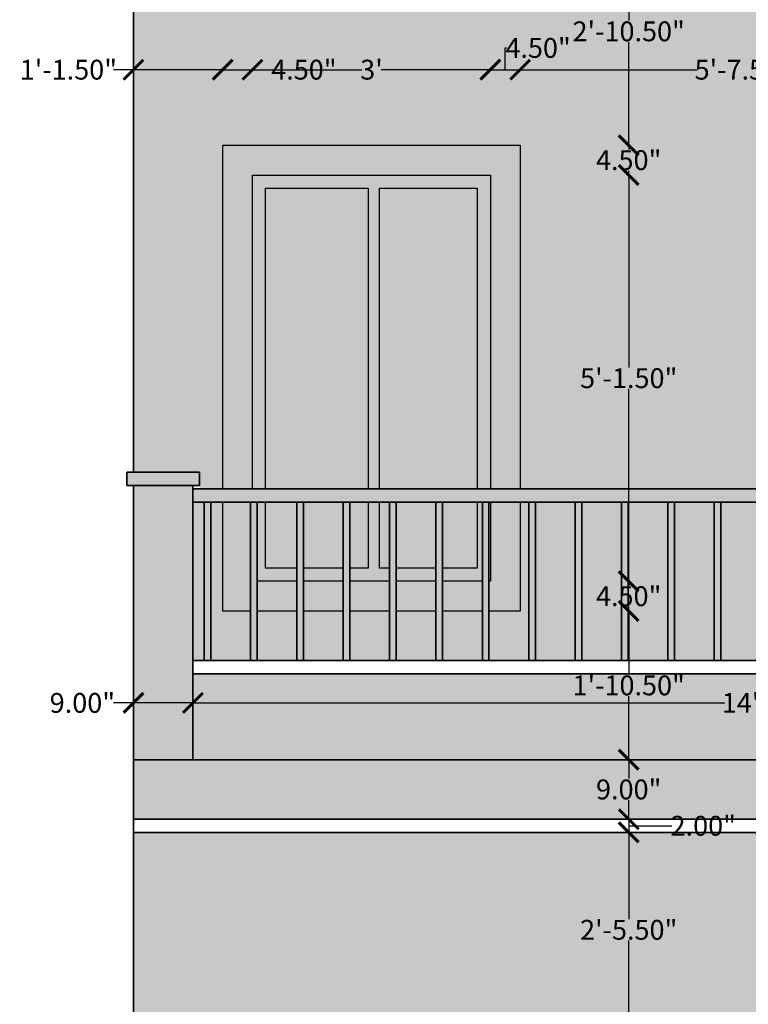
# Model space of a CAD drawing. Units: inches. Extents: x -654 to 390, y -40 to 648.
# Tile 10 of 13: x -19 to 92, y 417 to 566. Entities that reach past the tile are written whole.
import ezdxf

# ---------------------------------------------------------------- set-up
doc = ezdxf.new("R2010")
doc.units = ezdxf.units.IN
doc.header["$PDMODE"] = 3
for name, color, linetype, lineweight in [('A-ANNO-DIMS', 2, 'Continuous', 18), ('A-ELEV', 7, 'Continuous', 35), ('A-ELEV-FILL', 252, 'Continuous', 13), ('A-ELEV-PATT', 8, 'Continuous', 13), ('A-GLAZ', 4, 'Continuous', 25)]:
    doc.layers.add(name, color=color, linetype=linetype, lineweight=lineweight)
doc.styles.get("Standard").update_dxf_attribs({"font": 'arial.ttf'})
doc.dimstyles.get("Standard").update_dxf_attribs({"dimtxt": 3, "dimasz": 3, "dimexe": 0.18, "dimexo": 0.0625, "dimgap": 0.09, "dimtad": 0, "dimtih": 1, "dimtoh": 1, "dimzin": 0, "dimdsep": 46, "dimlunit": 3, "dimtxsty": 'Standard', "dimblk": 'ARCHTICK', "dimcen": 0.09, "dimse1": 1, "dimse2": 1, "dimadec": 0, "dimazin": 0, "dimtfac": 1, "dimtofl": 0, "dimtmove": 0, "dimatfit": 3, "dimfxl": 1, "dimtolj": 1, "dimtzin": 0, "dimarcsym": 0})

# ---------------------------------------------------------------- blocks, each defined once
blk = doc.blocks.new('_ArchTick')
at = {"color": 0, "linetype": 'ByBlock', "const_width": 0.15}
blk.add_lwpolyline([(-0.5, -0.5), (0.5, 0.5)], dxfattribs=at)
blk = doc.blocks.new('*D13')
at = {"layer": 'A-ANNO-DIMS', "color": 0, "lineweight": -2, "transparency": 16777216}
for p, q in [((73.57, 581.13), (73.57, 565.51)), ((73.57, 546.63), (73.57, 562.26))]:
    blk.add_line(p, q, dxfattribs=at)
at = {"layer": 'Defpoints', "color": 0, "transparency": 16777216}
for p in [(73.57, 581.13), (57.15, 546.63), (73.57, 546.63)]:
    blk.add_point(p, dxfattribs=at)
at = {"layer": 'A-ANNO-DIMS', "color": 0, "lineweight": -2, "transparency": 16777216, "xscale": 3, "yscale": 3, "zscale": 3}
for p, rotation in [((73.57, 581.13), 90), ((73.57, 546.63), 270)]:
    blk.add_blockref('_ArchTick', p, dxfattribs=dict(at, rotation=rotation))
at = {"layer": 'A-ANNO-DIMS', "color": 0, "transparency": 16777216, "insert": (73.57, 563.88), "char_height": 3, "attachment_point": 5}
blk.add_mtext('\\A1;2\'-10.50"', dxfattribs=at)
blk = doc.blocks.new('*D14')
at = {"layer": 'A-ANNO-DIMS', "color": 0, "lineweight": -2, "transparency": 16777216}
for p, q in [((73.57, 546.63), (73.57, 546.01)), ((73.57, 542.13), (73.57, 542.76))]:
    blk.add_line(p, q, dxfattribs=at)
at = {"layer": 'Defpoints', "color": 0, "transparency": 16777216}
for p in [(57.15, 546.63), (52.65, 542.13), (73.57, 542.13)]:
    blk.add_point(p, dxfattribs=at)
at = {"layer": 'A-ANNO-DIMS', "color": 0, "lineweight": -2, "transparency": 16777216, "xscale": 3, "yscale": 3, "zscale": 3}
for p, rotation in [((73.57, 546.63), 90), ((73.57, 542.13), 270)]:
    blk.add_blockref('_ArchTick', p, dxfattribs=dict(at, rotation=rotation))
at = {"layer": 'A-ANNO-DIMS', "color": 0, "transparency": 16777216, "insert": (73.57, 544.38), "char_height": 3, "attachment_point": 5}
blk.add_mtext('\\A1;4.50"', dxfattribs=at)
blk = doc.blocks.new('*D15')
at = {"layer": 'A-ANNO-DIMS', "color": 0, "lineweight": -2, "transparency": 16777216}
for p, q in [((73.57, 542.13), (73.57, 513.01)), ((73.57, 480.63), (73.57, 509.76))]:
    blk.add_line(p, q, dxfattribs=at)
at = {"layer": 'Defpoints', "color": 0, "transparency": 16777216}
for p in [(52.65, 542.13), (52.65, 480.63), (73.57, 480.63)]:
    blk.add_point(p, dxfattribs=at)
at = {"layer": 'A-ANNO-DIMS', "color": 0, "lineweight": -2, "transparency": 16777216, "xscale": 3, "yscale": 3, "zscale": 3}
for p, rotation in [((73.57, 542.13), 90), ((73.57, 480.63), 270)]:
    blk.add_blockref('_ArchTick', p, dxfattribs=dict(at, rotation=rotation))
at = {"layer": 'A-ANNO-DIMS', "color": 0, "transparency": 16777216, "insert": (73.57, 511.38), "char_height": 3, "attachment_point": 5}
blk.add_mtext('\\A1;5\'-1.50"', dxfattribs=at)
blk = doc.blocks.new('*D16')
at = {"layer": 'A-ANNO-DIMS', "color": 0, "lineweight": -2, "transparency": 16777216}
for p, q in [((73.57, 480.63), (73.57, 480.01)), ((73.57, 476.13), (73.57, 476.76))]:
    blk.add_line(p, q, dxfattribs=at)
at = {"layer": 'Defpoints', "color": 0, "transparency": 16777216}
for p in [(52.65, 480.63), (54.79, 476.13), (73.57, 476.13)]:
    blk.add_point(p, dxfattribs=at)
at = {"layer": 'A-ANNO-DIMS', "color": 0, "lineweight": -2, "transparency": 16777216, "xscale": 3, "yscale": 3, "zscale": 3}
for p, rotation in [((73.57, 480.63), 90), ((73.57, 476.13), 270)]:
    blk.add_blockref('_ArchTick', p, dxfattribs=dict(at, rotation=rotation))
at = {"layer": 'A-ANNO-DIMS', "color": 0, "transparency": 16777216, "insert": (73.57, 478.38), "char_height": 3, "attachment_point": 5}
blk.add_mtext('\\A1;4.50"', dxfattribs=at)
blk = doc.blocks.new('*D17')
at = {"layer": 'A-ANNO-DIMS', "color": 0, "lineweight": -2, "transparency": 16777216}
for p, q in [((73.57, 476.13), (73.57, 466.51)), ((73.57, 453.63), (73.57, 463.26))]:
    blk.add_line(p, q, dxfattribs=at)
at = {"layer": 'Defpoints', "color": 0, "transparency": 16777216}
for p in [(54.79, 476.13), (73.57, 453.63), (73.57, 453.63)]:
    blk.add_point(p, dxfattribs=at)
at = {"layer": 'A-ANNO-DIMS', "color": 0, "lineweight": -2, "transparency": 16777216, "xscale": 3, "yscale": 3, "zscale": 3}
for p, rotation in [((73.57, 476.13), 90), ((73.57, 453.63), 270)]:
    blk.add_blockref('_ArchTick', p, dxfattribs=dict(at, rotation=rotation))
at = {"layer": 'A-ANNO-DIMS', "color": 0, "transparency": 16777216, "insert": (73.57, 464.88), "char_height": 3, "attachment_point": 5}
blk.add_mtext('\\A1;1\'-10.50"', dxfattribs=at)
blk = doc.blocks.new('*D18')
at = {"layer": 'A-ANNO-DIMS', "color": 0, "lineweight": -2, "transparency": 16777216}
for p, q in [((73.57, 453.63), (73.57, 450.76)), ((73.57, 444.63), (73.57, 447.51))]:
    blk.add_line(p, q, dxfattribs=at)
at = {"layer": 'Defpoints', "color": 0, "transparency": 16777216}
for p in [(73.57, 453.63), (73.19, 444.63), (73.57, 444.63)]:
    blk.add_point(p, dxfattribs=at)
at = {"layer": 'A-ANNO-DIMS', "color": 0, "lineweight": -2, "transparency": 16777216, "xscale": 3, "yscale": 3, "zscale": 3}
for p, rotation in [((73.57, 453.63), 90), ((73.57, 444.63), 270)]:
    blk.add_blockref('_ArchTick', p, dxfattribs=dict(at, rotation=rotation))
at = {"layer": 'A-ANNO-DIMS', "color": 0, "transparency": 16777216, "insert": (73.57, 449.13), "char_height": 3, "attachment_point": 5}
blk.add_mtext('\\A1;9.00"', dxfattribs=at)
blk = doc.blocks.new('*D19')
at = {"layer": 'A-ANNO-DIMS', "color": 0, "lineweight": -2, "transparency": 16777216}
for p, q in [((73.57, 444.63), (73.57, 442.63)), ((73.57, 443.63), (79.92, 443.63)), ((79.92, 443.63), (80.1, 443.63))]:
    blk.add_line(p, q, dxfattribs=at)
at = {"layer": 'Defpoints', "color": 0, "transparency": 16777216}
for p in [(73.19, 444.63), (73.57, 442.63), (73.57, 442.63)]:
    blk.add_point(p, dxfattribs=at)
at = {"layer": 'A-ANNO-DIMS', "color": 0, "lineweight": -2, "transparency": 16777216, "xscale": 3, "yscale": 3, "zscale": 3}
for p, rotation in [((73.57, 444.63), 90), ((73.57, 442.63), 270)]:
    blk.add_blockref('_ArchTick', p, dxfattribs=dict(at, rotation=rotation))
at = {"layer": 'A-ANNO-DIMS', "color": 0, "transparency": 16777216, "insert": (84.85, 443.63), "char_height": 3, "attachment_point": 5}
blk.add_mtext('\\A1;2.00"', dxfattribs=at)
blk = doc.blocks.new('*D20')
at = {"layer": 'A-ANNO-DIMS', "color": 0, "lineweight": -2, "transparency": 16777216}
for p, q in [((73.57, 442.63), (73.57, 429.51)), ((73.57, 413.13), (73.57, 426.26))]:
    blk.add_line(p, q, dxfattribs=at)
at = {"layer": 'Defpoints', "color": 0, "transparency": 16777216}
for p in [(73.57, 442.63), (57.15, 413.13), (73.57, 413.13)]:
    blk.add_point(p, dxfattribs=at)
at = {"layer": 'A-ANNO-DIMS', "color": 0, "lineweight": -2, "transparency": 16777216, "xscale": 3, "yscale": 3, "zscale": 3}
for p, rotation in [((73.57, 442.63), 90), ((73.57, 413.13), 270)]:
    blk.add_blockref('_ArchTick', p, dxfattribs=dict(at, rotation=rotation))
at = {"layer": 'A-ANNO-DIMS', "color": 0, "transparency": 16777216, "insert": (73.57, 427.88), "char_height": 3, "attachment_point": 5}
blk.add_mtext('\\A1;2\'-5.50"', dxfattribs=at)
blk = doc.blocks.new('*D25')
at = {"layer": 'A-ANNO-DIMS', "color": 0, "lineweight": -2, "transparency": 16777216}
for p, q in [((-1.35, 558.08), (-4.35, 558.08)), ((12.15, 558.08), (-1.35, 558.08))]:
    blk.add_line(p, q, dxfattribs=at)
at = {"layer": 'Defpoints', "color": 0, "transparency": 16777216}
for p in [(-1.35, 558.08), (-1.35, 546.63), (12.15, 546.63)]:
    blk.add_point(p, dxfattribs=at)
at = {"layer": 'A-ANNO-DIMS', "color": 0, "lineweight": -2, "transparency": 16777216, "xscale": 3, "yscale": 3, "zscale": 3, "rotation": 180}
blk.add_blockref('_ArchTick', (-1.35, 558.08), dxfattribs=at)
at = {"layer": 'A-ANNO-DIMS', "color": 0, "lineweight": -2, "transparency": 16777216, "xscale": 3, "yscale": 3, "zscale": 3}
blk.add_blockref('_ArchTick', (12.15, 558.08), dxfattribs=at)
at = {"layer": 'A-ANNO-DIMS', "color": 0, "transparency": 16777216, "insert": (-11.2, 558.08), "char_height": 3, "attachment_point": 5}
blk.add_mtext('\\A1;1\'-1.50"', dxfattribs=at)
blk = doc.blocks.new('*D26')
at = {"layer": 'A-ANNO-DIMS', "color": 0, "lineweight": -2, "transparency": 16777216}
for p, q in [((12.15, 558.08), (16.65, 558.08)), ((16.65, 558.08), (19.65, 558.08))]:
    blk.add_line(p, q, dxfattribs=at)
at = {"layer": 'Defpoints', "color": 0, "transparency": 16777216}
for p in [(16.65, 558.08), (12.15, 546.63), (16.65, 542.13)]:
    blk.add_point(p, dxfattribs=at)
at = {"layer": 'A-ANNO-DIMS', "color": 0, "lineweight": -2, "transparency": 16777216, "xscale": 3, "yscale": 3, "zscale": 3, "rotation": 180}
blk.add_blockref('_ArchTick', (12.15, 558.08), dxfattribs=at)
at = {"layer": 'A-ANNO-DIMS', "color": 0, "lineweight": -2, "transparency": 16777216, "xscale": 3, "yscale": 3, "zscale": 3}
blk.add_blockref('_ArchTick', (16.65, 558.08), dxfattribs=at)
at = {"layer": 'A-ANNO-DIMS', "color": 0, "transparency": 16777216, "insert": (24.43, 558.08), "char_height": 3, "attachment_point": 5}
blk.add_mtext('\\A1;4.50"', dxfattribs=at)
blk = doc.blocks.new('*D27')
at = {"layer": 'A-ANNO-DIMS', "color": 0, "lineweight": -2, "transparency": 16777216}
for p, q in [((16.65, 558.08), (33.18, 558.08)), ((52.65, 558.08), (36.12, 558.08))]:
    blk.add_line(p, q, dxfattribs=at)
at = {"layer": 'Defpoints', "color": 0, "transparency": 16777216}
for p in [(52.65, 558.08), (16.65, 542.13), (52.65, 542.13)]:
    blk.add_point(p, dxfattribs=at)
at = {"layer": 'A-ANNO-DIMS', "color": 0, "lineweight": -2, "transparency": 16777216, "xscale": 3, "yscale": 3, "zscale": 3, "rotation": 180}
blk.add_blockref('_ArchTick', (16.65, 558.08), dxfattribs=at)
at = {"layer": 'A-ANNO-DIMS', "color": 0, "lineweight": -2, "transparency": 16777216, "xscale": 3, "yscale": 3, "zscale": 3}
blk.add_blockref('_ArchTick', (52.65, 558.08), dxfattribs=at)
at = {"layer": 'A-ANNO-DIMS', "color": 0, "transparency": 16777216, "insert": (34.65, 558.08), "char_height": 3, "attachment_point": 5}
blk.add_mtext("\\A1;3'", dxfattribs=at)
blk = doc.blocks.new('*D28')
at = {"layer": 'A-ANNO-DIMS', "color": 0, "lineweight": -2, "transparency": 16777216}
for p, q in [((54.9, 558.08), (54.9, 561.37)), ((54.9, 561.37), (55.08, 561.37)), ((52.65, 558.08), (57.15, 558.08))]:
    blk.add_line(p, q, dxfattribs=at)
at = {"layer": 'Defpoints', "color": 0, "transparency": 16777216}
for p in [(57.15, 558.08), (57.15, 546.63), (52.65, 542.13)]:
    blk.add_point(p, dxfattribs=at)
at = {"layer": 'A-ANNO-DIMS', "color": 0, "lineweight": -2, "transparency": 16777216, "xscale": 3, "yscale": 3, "zscale": 3, "rotation": 180}
blk.add_blockref('_ArchTick', (52.65, 558.08), dxfattribs=at)
at = {"layer": 'A-ANNO-DIMS', "color": 0, "lineweight": -2, "transparency": 16777216, "xscale": 3, "yscale": 3, "zscale": 3}
blk.add_blockref('_ArchTick', (57.15, 558.08), dxfattribs=at)
at = {"layer": 'A-ANNO-DIMS', "color": 0, "transparency": 16777216, "insert": (59.86, 561.37), "char_height": 3, "attachment_point": 5}
blk.add_mtext('\\A1;4.50"', dxfattribs=at)
blk = doc.blocks.new('*D29')
at = {"layer": 'A-ANNO-DIMS', "color": 0, "lineweight": -2, "transparency": 16777216}
for p, q in [((57.15, 558.08), (83.91, 558.08)), ((124.65, 558.08), (97.89, 558.08))]:
    blk.add_line(p, q, dxfattribs=at)
at = {"layer": 'Defpoints', "color": 0, "transparency": 16777216}
for p in [(124.65, 558.08), (124.65, 558.08), (57.15, 546.63)]:
    blk.add_point(p, dxfattribs=at)
at = {"layer": 'A-ANNO-DIMS', "color": 0, "lineweight": -2, "transparency": 16777216, "xscale": 3, "yscale": 3, "zscale": 3, "rotation": 180}
blk.add_blockref('_ArchTick', (57.15, 558.08), dxfattribs=at)
at = {"layer": 'A-ANNO-DIMS', "color": 0, "lineweight": -2, "transparency": 16777216, "xscale": 3, "yscale": 3, "zscale": 3}
blk.add_blockref('_ArchTick', (124.65, 558.08), dxfattribs=at)
at = {"layer": 'A-ANNO-DIMS', "color": 0, "transparency": 16777216, "insert": (90.9, 558.08), "char_height": 3, "attachment_point": 5}
blk.add_mtext('\\A1;5\'-7.50"', dxfattribs=at)
blk = doc.blocks.new('*D30')
at = {"layer": 'A-ANNO-DIMS', "color": 0, "lineweight": -2, "transparency": 16777216}
for p, q in [((-1.35, 462.23), (-4.35, 462.23)), ((7.65, 462.23), (-1.35, 462.23))]:
    blk.add_line(p, q, dxfattribs=at)
at = {"layer": 'Defpoints', "color": 0, "transparency": 16777216}
for p in [(-1.35, 462.23), (-1.35, 453.63), (7.65, 453.63)]:
    blk.add_point(p, dxfattribs=at)
at = {"layer": 'A-ANNO-DIMS', "color": 0, "lineweight": -2, "transparency": 16777216, "xscale": 3, "yscale": 3, "zscale": 3, "rotation": 180}
blk.add_blockref('_ArchTick', (-1.35, 462.23), dxfattribs=at)
at = {"layer": 'A-ANNO-DIMS', "color": 0, "lineweight": -2, "transparency": 16777216, "xscale": 3, "yscale": 3, "zscale": 3}
blk.add_blockref('_ArchTick', (7.65, 462.23), dxfattribs=at)
at = {"layer": 'A-ANNO-DIMS', "color": 0, "transparency": 16777216, "insert": (-9.08, 462.23), "char_height": 3, "attachment_point": 5}
blk.add_mtext('\\A1;9.00"', dxfattribs=at)
blk = doc.blocks.new('*D31')
at = {"layer": 'A-ANNO-DIMS', "color": 0, "lineweight": -2, "transparency": 16777216}
for p, q in [((7.65, 462.23), (88.13, 462.23)), ((184.65, 462.23), (104.16, 462.23))]:
    blk.add_line(p, q, dxfattribs=at)
at = {"layer": 'Defpoints', "color": 0, "transparency": 16777216}
for p in [(7.65, 462.23), (184.65, 462.23), (184.65, 462.23)]:
    blk.add_point(p, dxfattribs=at)
at = {"layer": 'A-ANNO-DIMS', "color": 0, "lineweight": -2, "transparency": 16777216, "xscale": 3, "yscale": 3, "zscale": 3, "rotation": 180}
blk.add_blockref('_ArchTick', (7.65, 462.23), dxfattribs=at)
at = {"layer": 'A-ANNO-DIMS', "color": 0, "lineweight": -2, "transparency": 16777216, "xscale": 3, "yscale": 3, "zscale": 3}
blk.add_blockref('_ArchTick', (184.65, 462.23), dxfattribs=at)
at = {"layer": 'A-ANNO-DIMS', "color": 0, "transparency": 16777216, "insert": (96.15, 462.23), "char_height": 3, "attachment_point": 5}
blk.add_mtext('\\A1;14\'-9.00"', dxfattribs=at)
blk = doc.blocks.new('*D80')
at = {"layer": 'A-ANNO-DIMS', "color": 0, "lineweight": -2, "transparency": 16777216}
for p, q in [((11.65, 643.23), (25.15, 643.23)), ((25.15, 643.23), (28.15, 643.23))]:
    blk.add_line(p, q, dxfattribs=at)
at = {"layer": 'Defpoints', "color": 0, "transparency": 16777216}
for p in [(25.15, 643.23), (11.65, 20.08), (25.15, 20.08)]:
    blk.add_point(p, dxfattribs=at)
at = {"layer": 'A-ANNO-DIMS', "color": 0, "lineweight": -2, "transparency": 16777216, "xscale": 3, "yscale": 3, "zscale": 3, "rotation": 180}
blk.add_blockref('_ArchTick', (11.65, 643.23), dxfattribs=at)
at = {"layer": 'A-ANNO-DIMS', "color": 0, "lineweight": -2, "transparency": 16777216, "xscale": 3, "yscale": 3, "zscale": 3}
blk.add_blockref('_ArchTick', (25.15, 643.23), dxfattribs=at)
at = {"layer": 'A-ANNO-DIMS', "color": 0, "transparency": 16777216, "insert": (35.58, 643.23), "char_height": 3, "attachment_point": 5}
blk.add_mtext('\\A1;1\'-1 1/2"', dxfattribs=at)

msp = doc.modelspace()

# ---------------------------------------------------------------- hatches: boundary and pattern name
at = {"layer": 'A-ELEV-FILL'}
h = msp.add_hatch(color=256, dxfattribs=at)
h.dxf.hatch_style = 1
h.paths.add_polyline_path([(126.646, 611.134), (124.646, 611.134), (-1.354, 611.134), (-3.354, 611.134), (-3.354, 609.134), (-1.354, 609.134), (124.646, 609.134), (126.646, 609.134)])
h.paths.add_polyline_path([(8.646, 497.134), (-2.354, 497.134), (-2.354, 495.134), (8.646, 495.134)])
h.paths.add_polyline_path([(346.646, 497.134), (182.515, 497.134), (182.515, 495.134), (346.646, 495.134)])
h.paths.add_polyline_path([(198.646, 486.134), (198.646, 473.634), (209.366, 474.634), (199.646, 474.634), (199.646, 485.134), (209.366, 485.134)])
h.paths.add_polyline_path([(332.646, 486.134), (198.646, 486.134), (209.366, 485.134), (321.926, 485.134)])
h.paths.add_polyline_path([(321.926, 474.634), (209.366, 474.634), (198.646, 473.634), (332.646, 473.634)])
h.paths.add_polyline_path([(332.646, 486.134), (321.926, 485.134), (331.646, 485.134), (331.646, 474.634), (321.926, 474.634), (332.646, 473.634)])
h = msp.add_hatch(color=256, dxfattribs=at)
h.dxf.hatch_style = 1
h.paths.add_polyline_path([(115.646, 305.634), (97.646, 305.634), (97.646, 306.634), (98.293, 306.634), (98.293, 315.634), (97.646, 315.634), (97.646, 316.634), (100.646, 316.634), (100.646, 442.634), (-1.354, 442.634), (-1.354, 125.134), (115.646, 125.134)])
h.paths.add_polyline_path([(57.146, 161.134), (12.146, 161.134), (12.146, 413.134), (57.146, 413.134)], flags=16)
h.paths.add_polyline_path([(52.646, 165.634), (16.646, 165.634), (16.646, 408.634), (52.646, 408.634)], flags=0)
h.paths.add_polyline_path([(52.146, 166.134), (17.146, 166.134), (17.146, 408.134), (52.146, 408.134)], flags=0)
h.paths.add_polyline_path([(124.646, 581.134), (-1.354, 581.134), (-1.354, 497.134), (8.646, 497.134), (8.646, 494.634), (12.146, 494.634), (12.146, 546.634), (57.146, 546.634), (57.146, 494.634), (124.646, 494.634)])
h.paths.add_polyline_path([(124.646, 609.134), (-1.354, 609.134), (-1.354, 590.134), (124.646, 590.134)])
h = msp.add_hatch(color=256, dxfattribs=at)
h.dxf.hatch_style = 1
h.paths.add_polyline_path([(161.035, 590.134), (-1.354, 590.134), (-1.354, 581.134), (161.035, 581.134)])
h.paths.add_polyline_path([(346.646, 453.634), (-1.354, 453.634), (-1.354, 444.634), (337.646, 444.634), (337.646, 177.634), (178.742, 177.634), (178.742, 173.134), (176.742, 173.134), (176.742, 177.634), (166.742, 177.634), (166.742, 173.134), (164.742, 173.134), (164.742, 177.634), (154.742, 177.634), (154.742, 173.134), (152.742, 173.134), (152.742, 177.634), (142.742, 177.634), (142.742, 173.134), (140.742, 173.134), (140.742, 177.634), (130.742, 177.634), (130.742, 173.134), (128.742, 173.134), (128.742, 177.634), (115.646, 177.634), (115.646, 168.634), (346.646, 168.634), (346.646, 173.134)])
h.paths.add_polyline_path([(7.646, 87.642), (-1.354, 87.642), (-1.354, 17.134), (7.646, 17.134)])
h.paths.add_polyline_path([(16.396, 116.134), (60.646, 116.134), (60.646, 83.134), (62.646, 83.134), (113.646, 83.134), (115.646, 83.134), (115.646, 125.134), (7.646, 125.134), (7.646, 89.642), (8.146, 89.642), (8.146, 87.642), (7.646, 87.642), (7.646, 83.134), (9.646, 83.134), (16.396, 83.134)])
h = msp.add_hatch(color=256, dxfattribs=at)
h.dxf.hatch_style = 1
h.paths.add_polyline_path([(57.146, 546.634), (12.146, 546.634), (12.146, 494.634), (16.646, 494.634), (16.646, 542.134), (52.646, 542.134), (52.646, 494.634), (57.146, 494.634)])
h.paths.add_polyline_path([(16.352, 492.634), (12.146, 492.634), (12.146, 476.134), (16.352, 476.134)])
h.paths.add_polyline_path([(23.368, 480.634), (17.352, 480.634), (17.352, 476.134), (23.368, 476.134)])
h.paths.add_polyline_path([(30.384, 480.634), (24.368, 480.634), (24.368, 476.134), (30.384, 476.134)])
h.paths.add_polyline_path([(37.4, 480.634), (31.384, 480.634), (31.384, 476.134), (37.4, 476.134)])
h.paths.add_polyline_path([(44.416, 480.634), (38.4, 480.634), (38.4, 476.134), (44.416, 476.134)])
h.paths.add_polyline_path([(51.432, 480.634), (45.416, 480.634), (45.416, 476.134), (51.432, 476.134)])
h.paths.add_polyline_path([(57.146, 492.634), (52.646, 492.634), (52.646, 480.634), (52.432, 480.634), (52.432, 476.134), (57.146, 476.134)])
h = msp.add_hatch(color=256, dxfattribs=at)
h.dxf.hatch_style = 1
h.paths.add_polyline_path([(52.646, 542.134), (16.646, 542.134), (16.646, 494.634), (18.646, 494.634), (18.646, 540.134), (34.168, 540.134), (34.168, 494.634), (35.875, 494.634), (35.875, 540.134), (50.651, 540.134), (50.651, 494.634), (52.646, 494.634)])
h.paths.add_polyline_path([(52.646, 492.634), (52.432, 492.634), (52.432, 480.634), (52.646, 480.634)])
h.paths.add_polyline_path([(51.432, 492.634), (50.651, 492.634), (50.651, 482.634), (45.416, 482.634), (45.416, 480.634), (51.432, 480.634)])
h.paths.add_polyline_path([(44.416, 482.634), (38.4, 482.634), (38.4, 480.634), (44.416, 480.634)])
h.paths.add_polyline_path([(37.4, 482.634), (35.875, 482.634), (35.875, 492.634), (34.168, 492.634), (34.168, 482.634), (31.384, 482.634), (31.384, 480.634), (37.4, 480.634)])
h.paths.add_polyline_path([(30.384, 482.634), (24.368, 482.634), (24.368, 480.634), (30.384, 480.634)])
h.paths.add_polyline_path([(23.368, 482.634), (18.646, 482.634), (18.646, 492.634), (17.352, 492.634), (17.352, 480.634), (23.368, 480.634)])
h = msp.add_hatch(color=256, dxfattribs=at)
h.dxf.hatch_style = 1
h.paths.add_polyline_path([(7.646, 495.134), (-1.354, 495.134), (-1.354, 453.634), (7.646, 453.634)])
h = msp.add_hatch(color=256, dxfattribs=at)
h.dxf.hatch_style = 1
h.paths.add_polyline_path([(295.646, 190.634), (178.742, 190.634), (178.742, 177.634), (295.646, 177.634)])
h.paths.add_polyline_path([(176.742, 190.634), (166.742, 190.634), (166.742, 177.634), (176.742, 177.634)])
h.paths.add_polyline_path([(164.742, 190.634), (154.742, 190.634), (154.742, 177.634), (164.742, 177.634)])
h.paths.add_polyline_path([(152.742, 190.634), (142.742, 190.634), (142.742, 177.634), (152.742, 177.634)])
h.paths.add_polyline_path([(140.742, 190.634), (130.742, 190.634), (130.742, 177.634), (140.742, 177.634)])
h.paths.add_polyline_path([(128.742, 190.634), (120.146, 190.634), (120.146, 177.634), (128.742, 177.634)])
h.paths.add_polyline_path([(295.646, 329.634), (145.646, 329.634), (145.646, 442.634), (100.646, 442.634), (100.646, 316.634), (295.646, 316.634)])
h.paths.add_polyline_path([(138.646, 359.634), (107.646, 359.634), (107.646, 438.634), (138.646, 438.634)], flags=16)
h.paths.add_polyline_path([(136.646, 361.634), (109.646, 361.634), (109.646, 436.634), (136.646, 436.634)], flags=0)
h.paths.add_polyline_path([(184.646, 466.634), (7.646, 466.634), (7.646, 453.634), (184.646, 453.634)])
h.paths.add_polyline_path([(184.646, 494.634), (7.646, 494.634), (7.646, 492.634), (184.646, 492.634)])
h.paths.add_polyline_path([(10.336, 492.634), (9.336, 492.634), (9.336, 468.634), (10.336, 468.634)])
h.paths.add_polyline_path([(17.352, 492.634), (16.352, 492.634), (16.352, 468.634), (17.352, 468.634)])
h.paths.add_polyline_path([(24.368, 492.634), (23.368, 492.634), (23.368, 468.634), (24.368, 468.634)])
h.paths.add_polyline_path([(31.384, 492.634), (30.384, 492.634), (30.384, 468.634), (31.384, 468.634)])
h.paths.add_polyline_path([(38.4, 492.634), (37.4, 492.634), (37.4, 468.634), (38.4, 468.634)])
h.paths.add_polyline_path([(45.416, 492.634), (44.416, 492.634), (44.416, 468.634), (45.416, 468.634)])
h.paths.add_polyline_path([(52.432, 492.634), (51.432, 492.634), (51.432, 468.634), (52.432, 468.634)])
h.paths.add_polyline_path([(59.448, 492.634), (58.448, 492.634), (58.448, 468.634), (59.448, 468.634)])
h.paths.add_polyline_path([(66.464, 492.634), (65.464, 492.634), (65.464, 468.634), (66.464, 468.634)])
h.paths.add_polyline_path([(73.48, 492.634), (72.48, 492.634), (72.48, 468.634), (73.48, 468.634)])
h.paths.add_polyline_path([(80.496, 492.634), (79.496, 492.634), (79.496, 468.634), (80.496, 468.634)])
h.paths.add_polyline_path([(87.512, 492.634), (86.512, 492.634), (86.512, 468.634), (87.512, 468.634)])
h.paths.add_polyline_path([(94.528, 492.634), (93.528, 492.634), (93.528, 468.634), (94.528, 468.634)])
h.paths.add_polyline_path([(101.544, 492.634), (100.544, 492.634), (100.544, 468.634), (101.544, 468.634)])
h.paths.add_polyline_path([(108.559, 492.634), (107.559, 492.634), (107.559, 468.634), (108.559, 468.634)])
h.paths.add_polyline_path([(115.575, 492.634), (114.575, 492.634), (114.575, 468.634), (115.575, 468.634)])
h.paths.add_polyline_path([(122.591, 492.634), (121.591, 492.634), (121.591, 468.634), (122.591, 468.634)])
h.paths.add_polyline_path([(129.607, 492.634), (128.607, 492.634), (128.607, 468.634), (129.607, 468.634)])
h.paths.add_polyline_path([(136.623, 492.634), (135.623, 492.634), (135.623, 468.634), (136.623, 468.634)])
h.paths.add_polyline_path([(143.639, 492.634), (142.639, 492.634), (142.639, 468.634), (143.639, 468.634)])
h.paths.add_polyline_path([(150.655, 492.634), (149.655, 492.634), (149.655, 468.634), (150.655, 468.634)])
h.paths.add_polyline_path([(157.671, 492.634), (156.671, 492.634), (156.671, 468.634), (157.671, 468.634)])
h.paths.add_polyline_path([(164.687, 492.634), (163.687, 492.634), (163.687, 468.634), (164.687, 468.634)])
h.paths.add_polyline_path([(171.703, 492.634), (170.703, 492.634), (170.703, 468.634), (171.703, 468.634)])
h.paths.add_polyline_path([(178.719, 492.634), (177.719, 492.634), (177.719, 468.634), (178.719, 468.634)])
h = msp.add_hatch(color=256, dxfattribs=at)
h.dxf.hatch_style = 1
h.paths.add_polyline_path([(121.591, 492.634), (115.575, 492.634), (115.575, 468.634), (121.591, 468.634)])
h.paths.add_polyline_path([(114.575, 492.634), (108.559, 492.634), (108.559, 468.634), (114.575, 468.634)])
h.paths.add_polyline_path([(107.559, 492.634), (101.544, 492.634), (101.544, 468.634), (107.559, 468.634)])
h.paths.add_polyline_path([(100.544, 492.634), (94.528, 492.634), (94.528, 468.634), (100.544, 468.634)])
h.paths.add_polyline_path([(93.528, 492.634), (87.512, 492.634), (87.512, 468.634), (93.528, 468.634)])
h.paths.add_polyline_path([(86.512, 492.634), (80.496, 492.634), (80.496, 468.634), (86.512, 468.634)])
h.paths.add_polyline_path([(79.496, 492.634), (73.48, 492.634), (73.48, 468.634), (79.496, 468.634)])
h.paths.add_polyline_path([(72.48, 492.634), (66.464, 492.634), (66.464, 468.634), (72.48, 468.634)])
h.paths.add_polyline_path([(65.464, 492.634), (59.448, 492.634), (59.448, 468.634), (65.464, 468.634)])
h.paths.add_polyline_path([(58.448, 492.634), (57.146, 492.634), (57.146, 476.134), (52.432, 476.134), (52.432, 468.634), (58.448, 468.634)])
h.paths.add_polyline_path([(51.432, 476.134), (45.416, 476.134), (45.416, 468.634), (51.432, 468.634)])
h.paths.add_polyline_path([(44.416, 476.134), (38.4, 476.134), (38.4, 468.634), (44.416, 468.634)])
h.paths.add_polyline_path([(37.4, 476.134), (31.384, 476.134), (31.384, 468.634), (37.4, 468.634)])
h.paths.add_polyline_path([(30.384, 476.134), (24.368, 476.134), (24.368, 468.634), (30.384, 468.634)])
h.paths.add_polyline_path([(23.368, 476.134), (17.352, 476.134), (17.352, 468.634), (23.368, 468.634)])
h.paths.add_polyline_path([(16.352, 476.134), (12.146, 476.134), (12.146, 492.634), (10.336, 492.634), (10.336, 468.634), (16.352, 468.634)])
h.paths.add_polyline_path([(9.336, 492.634), (7.646, 492.634), (7.646, 468.634), (9.336, 468.634)])
at = {"layer": 'A-ELEV-PATT'}
h = msp.add_hatch(dxfattribs=at)
h.set_pattern_fill('GOST_GLASS', color=256)
h.paths.add_polyline_path([(34.168, 540.134), (18.646, 540.134), (18.646, 494.634), (34.168, 494.634)])
h.paths.add_polyline_path([(50.651, 540.134), (35.875, 540.134), (35.875, 494.634), (50.651, 494.634)])
h.paths.add_polyline_path([(23.368, 492.634), (18.646, 492.634), (18.646, 482.634), (23.368, 482.634)])
h.paths.add_polyline_path([(30.384, 492.634), (24.368, 492.634), (24.368, 482.634), (30.384, 482.634)])
h.paths.add_polyline_path([(34.168, 492.634), (31.384, 492.634), (31.384, 482.634), (34.168, 482.634)])
h.paths.add_polyline_path([(44.416, 492.634), (38.4, 492.634), (38.4, 482.634), (44.416, 482.634)])
h.paths.add_polyline_path([(50.651, 492.634), (45.416, 492.634), (45.416, 482.634), (50.651, 482.634)])
h.paths.add_polyline_path([(37.4, 492.634), (35.875, 492.634), (35.875, 482.634), (37.4, 482.634)])
h.paths.add_polyline_path([(52.146, 408.134), (17.146, 408.134), (17.146, 360.234), (52.146, 360.234)])
h.paths.add_polyline_path([(52.146, 359.234), (17.146, 359.234), (17.146, 311.834), (52.146, 311.834)])
h.paths.add_polyline_path([(52.146, 310.834), (17.146, 310.834), (17.146, 263.434), (52.146, 263.434)])
h.paths.add_polyline_path([(52.146, 262.434), (17.146, 262.434), (17.146, 215.034), (52.146, 215.034)])
h.paths.add_polyline_path([(52.146, 214.034), (17.146, 214.034), (17.146, 166.134), (52.146, 166.134)])
h.paths.add_polyline_path([(44.556, 113.134), (33.082, 113.134), (33.082, 83.134), (44.556, 83.134)])
h.paths.add_polyline_path([(29.904, 113.134), (18.431, 113.134), (18.431, 83.134), (29.904, 83.134)])
h.paths.add_polyline_path([(59.143, 113.134), (47.67, 113.134), (47.67, 83.134), (59.143, 83.134)])
h.paths.add_polyline_path([(152.862, 134.63), (137.362, 134.63), (137.362, 74.63), (152.862, 74.63)])
h.paths.add_polyline_path([(170.362, 134.63), (154.862, 134.63), (154.862, 74.63), (170.362, 74.63)])
h.paths.add_polyline_path([(187.858, 134.63), (172.358, 134.63), (172.358, 74.63), (187.858, 74.63)])

# ---------------------------------------------------------------- linework, layer by layer
at = {"layer": 'A-ELEV'}
for p, q in [((-1.354, 497.134), (-1.354, 609.134)), ((-2.354, 497.134), (8.646, 497.134)), ((-2.354, 497.134), (-2.354, 495.134)), ((8.646, 495.134), (8.646, 497.134)), ((-2.354, 495.134), (8.646, 495.134)), ((-1.354, 89.642), (-1.354, 495.134)), ((7.646, 453.634), (7.646, 495.134)), ((7.646, 494.634), (184.646, 494.634)), ((7.646, 492.634), (184.646, 492.634)), ((9.336, 492.634), (9.336, 468.634)), ((10.336, 492.634), (10.336, 468.634)), ((16.352, 492.634), (16.352, 468.634)), ((17.352, 492.634), (17.352, 468.634)), ((23.368, 492.634), (23.368, 468.634)), ((24.368, 492.634), (24.368, 468.634)), ((30.384, 492.634), (30.384, 468.634)), ((31.384, 492.634), (31.384, 468.634)), ((37.4, 492.634), (37.4, 468.634)), ((38.4, 492.634), (38.4, 468.634)), ((44.416, 492.634), (44.416, 468.634)), ((45.416, 492.634), (45.416, 468.634)), ((51.432, 492.634), (51.432, 468.634)), ((52.432, 492.634), (52.432, 468.634)), ((58.448, 492.634), (58.448, 468.634)), ((59.448, 492.634), (59.448, 468.634)), ((65.464, 492.634), (65.464, 468.634)), ((66.464, 492.634), (66.464, 468.634)), ((72.48, 492.634), (72.48, 468.634)), ((73.48, 492.634), (73.48, 468.634)), ((79.496, 492.634), (79.496, 468.634)), ((80.496, 492.634), (80.496, 468.634)), ((86.512, 492.634), (86.512, 468.634)), ((87.512, 492.634), (87.512, 468.634)), ((7.646, 468.634), (184.646, 468.634)), ((7.646, 466.634), (184.646, 466.634)), ((-1.354, 453.634), (346.646, 453.634)), ((7.646, 453.634), (184.646, 453.634)), ((-1.354, 444.634), (337.646, 444.634)), ((-1.354, 442.634), (337.646, 442.634))]:
    msp.add_line(p, q, dxfattribs=at)
at = {"layer": 'A-GLAZ'}
for points in [[(12.146, 494.634), (12.146, 546.634), (57.146, 546.634), (57.146, 494.634)], [(16.646, 494.634), (16.646, 542.134), (52.646, 542.134), (52.646, 494.634)], [(18.646, 494.634), (18.646, 540.134), (34.168, 540.134), (34.168, 494.634)], [(35.875, 494.634), (35.875, 540.134), (50.651, 540.134), (50.651, 494.634)], [(16.352, 476.134), (12.146, 476.134), (12.146, 492.634)], [(23.368, 482.634), (18.646, 482.634), (18.646, 492.634)], [(34.168, 492.634), (34.168, 482.634), (31.384, 482.634)], [(37.4, 482.634), (35.875, 482.634), (35.875, 492.634)], [(50.651, 492.634), (50.651, 482.634), (45.416, 482.634)], [(52.646, 492.634), (52.646, 480.634), (52.432, 480.634)], [(57.146, 492.634), (57.146, 476.134), (52.432, 476.134)], [(30.384, 482.634), (24.368, 482.634)], [(44.416, 482.634), (38.4, 482.634)], [(23.368, 480.634), (17.352, 480.634)], [(30.384, 480.634), (24.368, 480.634)], [(37.4, 480.634), (31.384, 480.634)], [(44.416, 480.634), (38.4, 480.634)], [(51.432, 480.634), (45.416, 480.634)], [(23.368, 476.134), (17.352, 476.134)], [(30.384, 476.134), (24.368, 476.134)], [(37.4, 476.134), (31.384, 476.134)], [(44.416, 476.134), (38.4, 476.134)], [(51.432, 476.134), (45.416, 476.134)]]:
    msp.add_lwpolyline(points, dxfattribs=at)

# ---------------------------------------------------------------- dimensions: what is measured, and where the dimension line sits
at = {"layer": 'A-ANNO-DIMS'}
for base, p1, p2, override, picture, middle in [((25.146, 643.234), (11.646, 20.08), (25.146, 20.08), {"dimdec": 1, "dimlfac": 1, "dimrnd": 0, "dimzin": 1, "dimdsep": 46, "dimlunit": 4, "dimfrac": 2}, '*D80', (35.578, 643.234)), ((57.146, 558.077), (52.646, 542.134), (57.146, 546.634), {"dimclrd": 0, "dimclre": 0, "dimclrt": 0, "dimtmove": 1}, '*D28', (55.166, 561.365)), ((-1.354, 558.077), (12.146, 546.634), (-1.354, 546.634), {"dimclrd": 0, "dimclre": 0, "dimclrt": 0}, '*D25', (-11.203, 558.077)), ((16.646, 558.077), (12.146, 546.634), (16.646, 542.134), {"dimclrd": 0, "dimclre": 0, "dimclrt": 0}, '*D26', (24.434, 558.077)), ((52.646, 558.077), (16.646, 542.134), (52.646, 542.134), {"dimclrd": 0, "dimclre": 0, "dimclrt": 0, "dimtmove": 1}, '*D27', (34.646, 558.077)), ((124.646, 558.077), (57.146, 546.634), (124.646, 558.077), {"dimclrd": 0, "dimclre": 0, "dimclrt": 0, "dimtmove": 1}, '*D29', (90.896, 558.077)), ((-1.354, 462.232), (7.646, 453.634), (-1.354, 453.634), {"dimclrd": 0, "dimclre": 0, "dimclrt": 0}, '*D30', (-9.081, 462.232)), ((184.646, 462.232), (7.646, 462.232), (184.646, 462.232), {"dimclrd": 0, "dimclre": 0, "dimclrt": 0}, '*D31', (96.146, 462.232))]:
    dim = msp.add_linear_dim(base=base, p1=p1, p2=p2, dimstyle='Standard', override=override, dxfattribs=at)
    dim.commit()
    dim.dimension.update_dxf_attribs({"geometry": picture, "text_midpoint": middle})
for base, p1, p2, picture, middle in [((73.566, 546.634), (73.566, 581.134), (57.146, 546.634), '*D13', (73.566, 563.884)), ((73.566, 542.134), (57.146, 546.634), (52.646, 542.134), '*D14', (73.566, 544.384)), ((73.566, 480.634), (52.646, 542.134), (52.646, 480.634), '*D15', (73.566, 511.384)), ((73.566, 476.134), (52.646, 480.634), (54.789, 476.134), '*D16', (73.566, 478.384)), ((73.566, 453.634), (54.789, 476.134), (73.566, 453.634), '*D17', (73.566, 464.884)), ((73.566, 444.634), (73.566, 453.634), (73.186, 444.634), '*D18', (73.566, 449.134)), ((73.566, 442.634), (73.186, 444.634), (73.566, 442.634), '*D19', (80.188, 443.634)), ((73.566, 413.134), (73.566, 442.634), (57.146, 413.134), '*D20', (73.566, 427.884))]:
    dim = msp.add_linear_dim(base=base, p1=p1, p2=p2, angle=90, dimstyle='Standard', override={"dimclrd": 0, "dimclre": 0, "dimclrt": 0, "dimtmove": 1}, dxfattribs=at)
    dim.commit()
    dim.dimension.update_dxf_attribs({"geometry": picture, "text_midpoint": middle})

doc.saveas('drawing.dxf')
